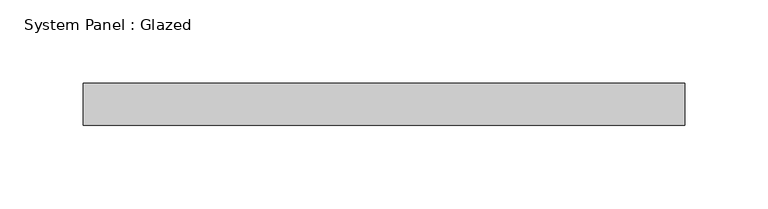
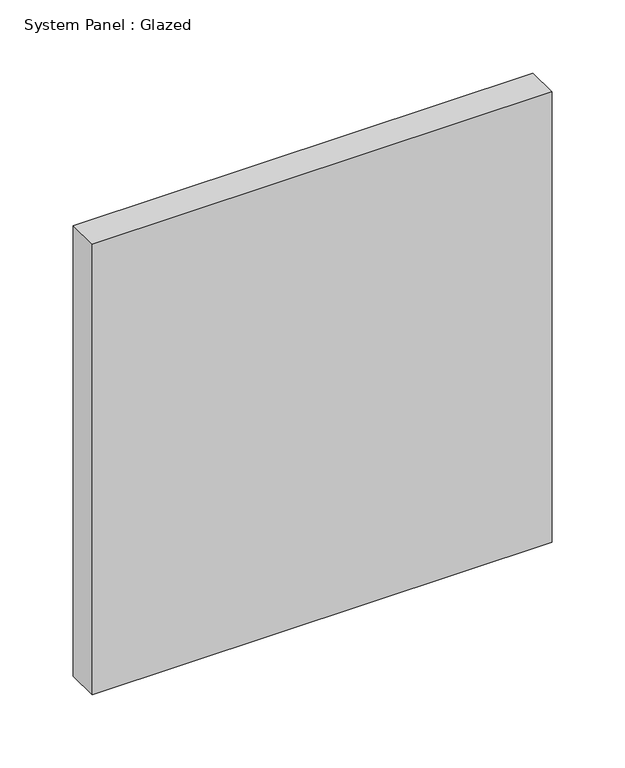
"""IFC4 building model written with IfcOpenShell, lengths in millimetres: plate geometry, System Panel : Glazed."""

from ifc_helpers import new_model, si_unit, origin, origin_with_axes, place, context, project, spatial, polyline, outline, extrude, source, transform, mapped, element, save


def system_panel_glazed_b1e52c84(model_context):
    return source(origin(), model_context, "Body", "SweptSolid", [
        extrude(outline(polyline([(180.975, 19.05), (-180.975, 19.05), (-180.975, 44.45), (180.975, 44.45), (180.975, 19.05)])), origin_with_axes(), (0.0, 0.0, 1.0), 374.65),
    ])


if __name__ == "__main__":
    model = new_model("IFC4")
    model_context = context("Model", 3, world=origin())
    ifc_project = project(units=[si_unit("LENGTHUNIT", "METRE", prefix="MILLI")], contexts=[model_context])
    site = spatial("IfcSite", under=ifc_project)
    building = spatial("IfcBuilding", under=site)
    placement = place(None, origin())
    system_panel_glazed_shape = system_panel_glazed_b1e52c84(model_context)
    element("IfcPlate", 1, ObjectType="System Panel : Glazed", at=placement, inside=building, context=model_context, shape_type="MappedRepresentation", body=[
        mapped(system_panel_glazed_shape, transform((0.0, 0.0, 0.0), x_axis=(1.0, 0.0, 0.0), y_axis=(0.0, 1.0, 0.0), z_axis=(0.0, 0.0, 1.0))),
    ])
    save(model, "model.ifc")

# Revit data of these elements
# Type "System Panel : Glazed"
#   Construction Type Id = "GSP4R"
#   Analytic Construction = "1/8 in Pilkington single glazing"
#   Visual Light Transmittance = 0.9
#   Solar Heat Gain Coefficient = 0.86
#   Heat Transfer Coefficient (U) = 1.18115 BTU/(h·ft²·°F)
#   Define Thermal Properties by = 1
# Element 1 (IfcPlate, "System Panel : Glazed")
#   Materials on its faces: "Glass"
# Materials
#   "Glass": class "Glass", colour RGB 0 128 192, transparency 0.75, Description = "Soda Lime Glass", Cost = 0
